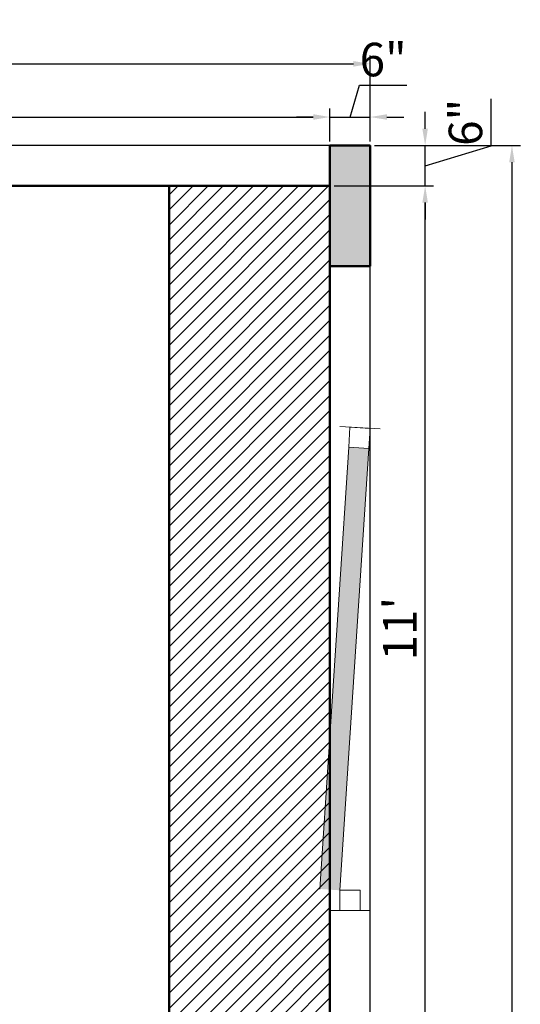
# Model space of a CAD drawing. Units: inches. Extents: x 3064 to 19385, y 846 to 15425.
# Tile 64 of 108: x 6332 to 6407, y 1860 to 2007. Entities that reach past the tile are written whole.
import ezdxf

# ---------------------------------------------------------------- set-up
doc = ezdxf.new("R2010")
doc.units = ezdxf.units.IN
for name, color, linetype, lineweight in [('A-ANNO-DIMS', 2, 'Continuous', 18), ('A-COLS', 1, 'Continuous', 35), ('A-FURN-PATT', 252, 'Continuous', 13), ('A-GLAZ', 4, 'Continuous', 18), ('A-WALL', 7, 'Continuous', 50), ('C-PROP', 6, 'Continuous', 25)]:
    doc.layers.add(name, color=color, linetype=linetype, lineweight=lineweight)
doc.styles.get("Standard").update_dxf_attribs({"font": 'arial.ttf'})
doc.dimstyles.new('ISO-25', dxfattribs={"dimtxt": 9, "dimasz": 2.5, "dimexe": 1.25, "dimexo": 0.625, "dimtad": 1, "dimdec": 1, "dimlunit": 3, "dimtxsty": 'Standard', "dimcen": 2.5, "dimadec": 0, "dimazin": 0, "dimtfac": 1, "dimtdec": 1, "dimtmove": 0, "dimatfit": 3, "dimfxl": 1, "dimarcsym": 0})

# ---------------------------------------------------------------- blocks, each defined once
blk = doc.blocks.new('*D387')
at = {"layer": 'A-ANNO-DIMS', "color": 0, "lineweight": -2, "transparency": 16777216}
for p, q in [((6183.49, 1988.61), (6183.49, 1993.49)), ((6378.49, 1988.61), (6378.49, 1993.49)), ((6185.99, 1992.24), (6375.99, 1992.24))]:
    blk.add_line(p, q, dxfattribs=at)
at = {"layer": 'A-ANNO-DIMS', "color": 0, "transparency": 16777216}
for points in [[(6185.99, 1992.66), (6185.99, 1991.83), (6183.49, 1992.24)], [(6375.99, 1992.66), (6375.99, 1991.83), (6378.49, 1992.24)]]:
    blk.add_solid(points, dxfattribs=at)
at = {"layer": 'Defpoints', "color": 0, "transparency": 16777216}
for p in [(6378.49, 1992.24), (6183.49, 1987.99), (6378.49, 1987.99)]:
    blk.add_point(p, dxfattribs=at)
at = {"layer": 'A-ANNO-DIMS', "color": 0, "transparency": 16777216, "insert": (6280.99, 1995.42), "char_height": 5, "attachment_point": 5}
blk.add_mtext('16\'-3"', dxfattribs=at)
blk = doc.blocks.new('*D388')
at = {"layer": 'A-ANNO-DIMS', "color": 0, "lineweight": -2, "transparency": 16777216}
for p, q in [((6381.49, 1992.24), (6382.91, 1996.98)), ((6382.91, 1996.98), (6389.94, 1996.98)), ((6378.49, 1988.61), (6378.49, 1993.49)), ((6384.49, 1988.61), (6384.49, 1993.49)), ((6375.99, 1992.24), (6373.49, 1992.24)), ((6378.49, 1992.24), (6384.49, 1992.24)), ((6378.49, 1992.24), (6384.49, 1992.24)), ((6386.99, 1992.24), (6389.49, 1992.24))]:
    blk.add_line(p, q, dxfattribs=at)
at = {"layer": 'A-ANNO-DIMS', "color": 0, "transparency": 16777216}
for points in [[(6375.99, 1992.66), (6375.99, 1991.83), (6378.49, 1992.24)], [(6386.99, 1992.66), (6386.99, 1991.83), (6384.49, 1992.24)]]:
    blk.add_solid(points, dxfattribs=at)
at = {"layer": 'Defpoints', "color": 0, "transparency": 16777216}
for p in [(6384.49, 1992.24), (6378.49, 1987.99), (6384.49, 1987.99)]:
    blk.add_point(p, dxfattribs=at)
at = {"layer": 'A-ANNO-DIMS', "color": 0, "transparency": 16777216, "insert": (6386.43, 2000.16), "char_height": 5, "attachment_point": 5}
blk.add_mtext('6"', dxfattribs=at)
blk = doc.blocks.new('*D375')
at = {"layer": 'A-ANNO-DIMS', "color": 0, "lineweight": -2, "transparency": 16777216}
for p, q in [((6379.12, 1981.99), (6393.94, 1981.99)), ((6392.69, 1852.49), (6392.69, 1979.49)), ((6385.12, 1849.99), (6393.94, 1849.99))]:
    blk.add_line(p, q, dxfattribs=at)
at = {"layer": 'A-ANNO-DIMS', "color": 0, "transparency": 16777216}
for points in [[(6392.27, 1979.49), (6393.1, 1979.49), (6392.69, 1981.99)], [(6392.27, 1852.49), (6393.1, 1852.49), (6392.69, 1849.99)]]:
    blk.add_solid(points, dxfattribs=at)
at = {"layer": 'Defpoints', "color": 0, "transparency": 16777216}
for p in [(6378.49, 1981.99), (6392.69, 1981.99), (6384.49, 1849.99)]:
    blk.add_point(p, dxfattribs=at)
at = {"layer": 'A-ANNO-DIMS', "color": 0, "transparency": 16777216, "insert": (6389.55, 1915.99), "char_height": 5, "attachment_point": 5, "rotation": 90}
blk.add_mtext("11'", dxfattribs=at)
blk = doc.blocks.new('*D376')
at = {"layer": 'A-ANNO-DIMS', "color": 0, "lineweight": -2, "transparency": 16777216}
for p, q in [((6402.53, 1987.94), (6402.53, 1994.97)), ((6392.69, 1990.49), (6392.69, 1992.99)), ((6385.12, 1987.99), (6393.94, 1987.99)), ((6392.69, 1981.99), (6392.69, 1987.99)), ((6392.69, 1981.99), (6392.69, 1987.99)), ((6392.69, 1984.99), (6402.53, 1987.94)), ((6379.12, 1981.99), (6393.94, 1981.99)), ((6392.69, 1979.49), (6392.69, 1976.99))]:
    blk.add_line(p, q, dxfattribs=at)
at = {"layer": 'A-ANNO-DIMS', "color": 0, "transparency": 16777216}
for points in [[(6392.27, 1990.49), (6393.1, 1990.49), (6392.69, 1987.99)], [(6392.27, 1979.49), (6393.1, 1979.49), (6392.69, 1981.99)]]:
    blk.add_solid(points, dxfattribs=at)
at = {"layer": 'Defpoints', "color": 0, "transparency": 16777216}
for p in [(6384.49, 1987.99), (6392.69, 1987.99), (6378.49, 1981.99)]:
    blk.add_point(p, dxfattribs=at)
at = {"layer": 'A-ANNO-DIMS', "color": 0, "transparency": 16777216, "insert": (6399.35, 1991.45), "char_height": 5, "attachment_point": 5, "rotation": 90}
blk.add_mtext('6"', dxfattribs=at)
blk = doc.blocks.new('*D377')
at = {"layer": 'A-ANNO-DIMS', "color": 0, "lineweight": -2, "transparency": 16777216}
for p, q in [((6385.12, 1987.99), (6406.89, 1987.99)), ((6405.64, 1985.49), (6405.64, 1474.49)), ((6385.12, 1471.99), (6406.89, 1471.99))]:
    blk.add_line(p, q, dxfattribs=at)
at = {"layer": 'A-ANNO-DIMS', "color": 0, "transparency": 16777216}
for points in [[(6405.22, 1985.49), (6406.05, 1985.49), (6405.64, 1987.99)], [(6405.22, 1474.49), (6406.05, 1474.49), (6405.64, 1471.99)]]:
    blk.add_solid(points, dxfattribs=at)
at = {"layer": 'Defpoints', "color": 0, "transparency": 16777216}
for p in [(6384.49, 1987.99), (6384.49, 1471.99), (6405.64, 1471.99)]:
    blk.add_point(p, dxfattribs=at)
at = {"layer": 'A-ANNO-DIMS', "color": 0, "transparency": 16777216, "insert": (6402.46, 1729.99), "char_height": 5, "attachment_point": 5, "rotation": 90}
blk.add_mtext("43'", dxfattribs=at)
blk = doc.blocks.new('*D378')
at = {"layer": 'A-ANNO-DIMS', "color": 0, "lineweight": -2, "transparency": 16777216}
for p, q in [((6042.49, 1988.61), (6042.49, 2001.41)), ((6044.99, 2000.16), (6381.99, 2000.16)), ((6384.49, 1988.61), (6384.49, 2001.41))]:
    blk.add_line(p, q, dxfattribs=at)
at = {"layer": 'A-ANNO-DIMS', "color": 0, "transparency": 16777216}
for points in [[(6044.99, 2000.58), (6044.99, 1999.75), (6042.49, 2000.16)], [(6381.99, 2000.58), (6381.99, 1999.75), (6384.49, 2000.16)]]:
    blk.add_solid(points, dxfattribs=at)
at = {"layer": 'Defpoints', "color": 0, "transparency": 16777216}
for p in [(6384.49, 2000.16), (6042.49, 1987.99), (6384.49, 1987.99)]:
    blk.add_point(p, dxfattribs=at)
at = {"layer": 'A-ANNO-DIMS', "color": 0, "transparency": 16777216, "insert": (6213.49, 2003.34), "char_height": 5, "attachment_point": 5}
blk.add_mtext('28\'-6"', dxfattribs=at)
blk = doc.blocks.new('WIN-1900-A')
h = blk.add_hatch(color=256)
h.dxf.hatch_style = 1
h.paths.add_polyline_path([(1.5, 0), (4.5, 0), (4.5, 66), (1.5, 66)])
for p, q in [((0, 69), (6, 69)), ((1.5, 66), (1.5, 0)), ((4.5, 66), (4.5, 0))]:
    blk.add_line(p, q)
blk.add_lwpolyline([(4.5, 66), (1.5, 66), (1.5, 69), (4.5, 69)], close=True)

msp = doc.modelspace()

# ---------------------------------------------------------------- hatches: boundary and pattern name
at = {"layer": 'A-COLS'}
h = msp.add_hatch(color=256, dxfattribs=at)
h.dxf.hatch_style = 1
h.paths.add_polyline_path([(6378.49, 1969.99), (6384.49, 1969.99), (6384.49, 1987.99), (6378.49, 1987.99)])
at = {"layer": 'A-FURN-PATT'}
h = msp.add_hatch(dxfattribs=at)
h.set_pattern_fill('ANSI31', color=256, scale=0.5)
h.set_pattern_definition([(45, (726.825, 591.649), (-1.122532, 1.122532), [])])
h.paths.add_polyline_path([(6354.49, 1849.99), (6378.49, 1849.99), (6378.49, 1981.99), (6354.49, 1981.99)])

# ---------------------------------------------------------------- linework, layer by layer
at = {"layer": 'A-GLAZ'}
msp.add_line((6384.49, 1873.99), (6378.49, 1873.99), dxfattribs=at)
msp.add_lwpolyline([(6382.99, 1873.99), (6379.99, 1873.99), (6379.99, 1876.99), (6382.99, 1876.99)], close=True, dxfattribs=at)
at = {"layer": 'A-WALL'}
for p, q in [((6378.49, 1981.99), (6183.49, 1981.99)), ((6354.49, 1843.99), (6354.49, 1981.99)), ((6378.49, 1849.99), (6378.49, 1981.99))]:
    msp.add_line(p, q, dxfattribs=at)
msp.add_lwpolyline([(6384.49, 1969.99), (6384.49, 1987.99), (6378.49, 1987.99), (6378.49, 1969.99)], close=True, dxfattribs=at)
at = {"layer": 'C-PROP'}
for p, q in [((6384.49, 1987.99), (6042.49, 1987.99)), ((6384.49, 1471.99), (6384.49, 1987.99))]:
    msp.add_line(p, q, dxfattribs=at)

# ---------------------------------------------------------------- block references
at = {"layer": 'A-GLAZ', "rotation": 356.2747581013879}
msp.add_blockref('WIN-1900-A', (6375.5, 1877.28), dxfattribs=at)

# ---------------------------------------------------------------- dimensions: what is measured, and where the dimension line sits
at = {"layer": 'A-ANNO-DIMS'}
for base, p1, p2, override, picture, middle in [((6384.49, 2000.16), (6042.49, 1987.99), (6384.49, 1987.99), {"dimtxt": 5, "dimclrd": 0, "dimclre": 0, "dimclrt": 0}, '*D378', (6213.49, 2003.34)), ((6384.49, 1992.24), (6378.49, 1987.99), (6384.49, 1987.99), {"dimtxt": 5, "dimclrd": 0, "dimclre": 0, "dimclrt": 0, "dimtmove": 1}, '*D388', (6383.54, 2000.16)), ((6378.49, 1992.24), (6183.49, 1987.99), (6378.49, 1987.99), {"dimtxt": 5, "dimclrd": 0, "dimclre": 0, "dimclrt": 0, "dimtmove": 1}, '*D387', (6280.99, 1995.42))]:
    dim = msp.add_linear_dim(base=base, p1=p1, p2=p2, dimstyle='ISO-25', override=override, dxfattribs=at)
    dim.commit()
    dim.dimension.update_dxf_attribs({"geometry": picture, "text_midpoint": middle})
for base, p1, p2, override, picture, middle in [((6392.69, 1987.99), (6378.49, 1981.99), (6384.49, 1987.99), {"dimtxt": 5, "dimclrd": 0, "dimclre": 0, "dimclrt": 0, "dimtmove": 1}, '*D376', (6399.35, 1988.57)), ((6405.64, 1471.99), (6384.49, 1987.99), (6384.49, 1471.99), {"dimtxt": 5, "dimclrd": 0, "dimclre": 0, "dimclrt": 0}, '*D377', (6402.46, 1729.99)), ((6392.69, 1981.99), (6384.49, 1849.99), (6378.49, 1981.99), {"dimtxt": 5, "dimclrd": 0, "dimclre": 0, "dimclrt": 0, "dimtmove": 1}, '*D375', (6389.55, 1915.99))]:
    dim = msp.add_linear_dim(base=base, p1=p1, p2=p2, angle=90, dimstyle='ISO-25', override=override, dxfattribs=at)
    dim.commit()
    dim.dimension.update_dxf_attribs({"geometry": picture, "text_midpoint": middle})

doc.saveas('drawing.dxf')
